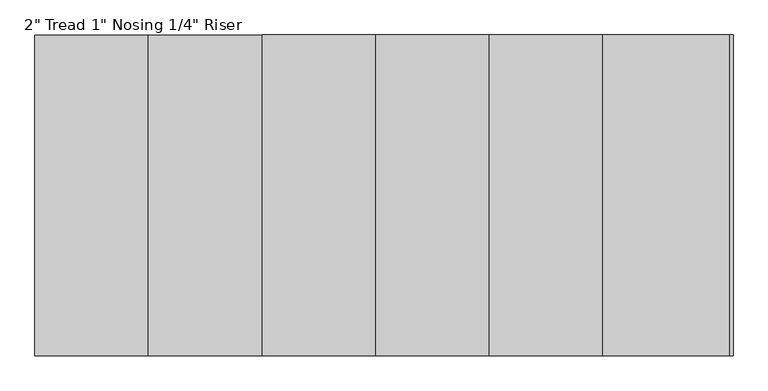
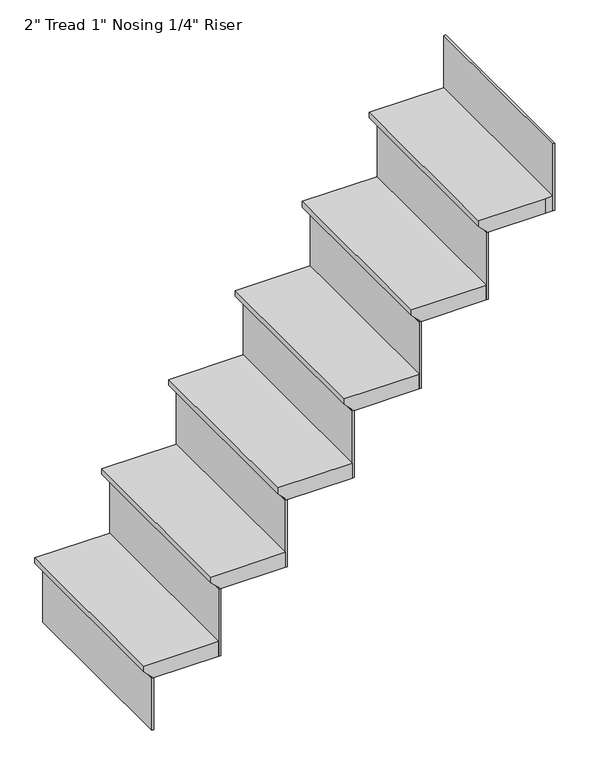
"""IFC4 building model written with IfcOpenShell, lengths in millimetres: stair flight geometry."""

from ifc_helpers import new_model, si_unit, origin, place, context, project, spatial, faceted_brep, source, transform, mapped, element, save


def stair_flight_6b27b35d(model_context):
    return source(origin(), model_context, "Body", "Brep", [
        faceted_brep([(-4591.4237097, 3724.9480625, 209.55), (-4591.4237097, 3724.9480625, 228.6), (-4591.4237097, 4334.5480625, 228.6), (-4591.4237097, 4334.5480625, 209.55), (-4566.0237097, 3724.9480625, 184.15), (-4566.0237097, 4334.5480625, 184.15), (-4350.1237097, 3724.9480625, 228.6), (-4350.1237097, 4334.5480625, 228.6), (-4566.0237097, 4334.5480625, 177.8), (-4350.1237097, 4334.5480625, 177.8), (-4350.1237097, 3724.9480625, 177.8), (-4566.0237097, 3724.9480625, 177.8)], [[[0, 1, 2, 3]], [[4, 0, 3, 5]], [[2, 1, 6, 7]], [[8, 9, 10, 11]], [[2, 7, 9, 8, 5, 3]], [[8, 11, 4, 5]], [[6, 1, 0, 4, 11, 10]], [[7, 6, 10, 9]]]),
        faceted_brep([(-4566.0237097, 3724.9480625, 177.8), (-4566.0237097, 3724.9480625, 0.0), (-4559.6737097, 3724.9480625, 0.0), (-4559.6737097, 3724.9480625, 177.8), (-4566.0237097, 4334.5480625, 177.8), (-4559.6737097, 4334.5480625, 177.8), (-4559.6737097, 4334.5480625, 0.0), (-4566.0237097, 4334.5480625, 0.0)], [[[0, 1, 2, 3]], [[4, 5, 6, 7]], [[1, 0, 4, 7]], [[2, 1, 7, 6]], [[3, 2, 6, 5]], [[0, 3, 5, 4]]]),
        faceted_brep([(-3270.6237097, 3724.9480625, 1549.4), (-3270.6237097, 3724.9480625, 1320.8), (-3264.2737097, 3724.9480625, 1320.8), (-3264.2737097, 3724.9480625, 1549.4), (-3270.6237097, 4334.5480625, 1549.4), (-3264.2737097, 4334.5480625, 1549.4), (-3264.2737097, 4334.5480625, 1320.8), (-3270.6237097, 4334.5480625, 1320.8)], [[[0, 1, 2, 3]], [[4, 5, 6, 7]], [[1, 0, 4, 7]], [[2, 1, 7, 6]], [[3, 2, 6, 5]], [[0, 3, 5, 4]]]),
        faceted_brep([(-4350.1237097, 3724.9480625, 406.4), (-4350.1237097, 3724.9480625, 177.8), (-4343.7737097, 3724.9480625, 177.8), (-4343.7737097, 3724.9480625, 406.4), (-4350.1237097, 4334.5480625, 406.4), (-4343.7737097, 4334.5480625, 406.4), (-4343.7737097, 4334.5480625, 177.8), (-4350.1237097, 4334.5480625, 177.8)], [[[0, 1, 2, 3]], [[4, 5, 6, 7]], [[1, 0, 4, 7]], [[2, 1, 7, 6]], [[3, 2, 6, 5]], [[0, 3, 5, 4]]]),
        faceted_brep([(-4375.5237097, 4334.5480625, 457.2), (-4375.5237097, 3724.9480625, 457.2), (-4134.2237097, 3724.9480625, 457.2), (-4134.2237097, 4334.5480625, 457.2), (-4350.1237097, 4334.5480625, 406.4), (-4134.2237097, 4334.5480625, 406.4), (-4134.2237097, 3724.9480625, 406.4), (-4350.1237097, 3724.9480625, 406.4), (-4350.1237097, 4334.5480625, 412.75), (-4375.5237097, 4334.5480625, 438.15), (-4350.1237097, 3724.9480625, 412.75), (-4375.5237097, 3724.9480625, 438.15)], [[[0, 1, 2, 3]], [[4, 5, 6, 7]], [[0, 3, 5, 4, 8, 9]], [[4, 7, 10, 8]], [[2, 1, 11, 10, 7, 6]], [[3, 2, 6, 5]], [[11, 1, 0, 9]], [[10, 11, 9, 8]]]),
        faceted_brep([(-4134.2237097, 3724.9480625, 635.0), (-4134.2237097, 3724.9480625, 406.4), (-4127.8737097, 3724.9480625, 406.4), (-4127.8737097, 3724.9480625, 635.0), (-4134.2237097, 4334.5480625, 635.0), (-4127.8737097, 4334.5480625, 635.0), (-4127.8737097, 4334.5480625, 406.4), (-4134.2237097, 4334.5480625, 406.4)], [[[0, 1, 2, 3]], [[4, 5, 6, 7]], [[1, 0, 4, 7]], [[2, 1, 7, 6]], [[3, 2, 6, 5]], [[0, 3, 5, 4]]]),
        faceted_brep([(-4159.6237097, 4334.5480625, 685.8), (-4159.6237097, 3724.9480625, 685.8), (-3918.3237097, 3724.9480625, 685.8), (-3918.3237097, 4334.5480625, 685.8), (-4134.2237097, 4334.5480625, 635.0), (-3918.3237097, 4334.5480625, 635.0), (-3918.3237097, 3724.9480625, 635.0), (-4134.2237097, 3724.9480625, 635.0), (-4134.2237097, 4334.5480625, 641.35), (-4159.6237097, 4334.5480625, 666.75), (-4134.2237097, 3724.9480625, 641.35), (-4159.6237097, 3724.9480625, 666.75)], [[[0, 1, 2, 3]], [[4, 5, 6, 7]], [[0, 3, 5, 4, 8, 9]], [[4, 7, 10, 8]], [[2, 1, 11, 10, 7, 6]], [[3, 2, 6, 5]], [[11, 1, 0, 9]], [[10, 11, 9, 8]]]),
        faceted_brep([(-3918.3237097, 3724.9480625, 863.6), (-3918.3237097, 3724.9480625, 635.0), (-3911.9737097, 3724.9480625, 635.0), (-3911.9737097, 3724.9480625, 863.6), (-3918.3237097, 4334.5480625, 863.6), (-3911.9737097, 4334.5480625, 863.6), (-3911.9737097, 4334.5480625, 635.0), (-3918.3237097, 4334.5480625, 635.0)], [[[0, 1, 2, 3]], [[4, 5, 6, 7]], [[1, 0, 4, 7]], [[2, 1, 7, 6]], [[3, 2, 6, 5]], [[0, 3, 5, 4]]]),
        faceted_brep([(-3943.7237097, 4334.5480625, 914.4), (-3943.7237097, 3724.9480625, 914.4), (-3702.4237097, 3724.9480625, 914.4), (-3702.4237097, 4334.5480625, 914.4), (-3918.3237097, 4334.5480625, 863.6), (-3702.4237097, 4334.5480625, 863.6), (-3702.4237097, 3724.9480625, 863.6), (-3918.3237097, 3724.9480625, 863.6), (-3918.3237097, 4334.5480625, 869.95), (-3943.7237097, 4334.5480625, 895.35), (-3918.3237097, 3724.9480625, 869.95), (-3943.7237097, 3724.9480625, 895.35)], [[[0, 1, 2, 3]], [[4, 5, 6, 7]], [[0, 3, 5, 4, 8, 9]], [[4, 7, 10, 8]], [[2, 1, 11, 10, 7, 6]], [[3, 2, 6, 5]], [[11, 1, 0, 9]], [[10, 11, 9, 8]]]),
        faceted_brep([(-3702.4237097, 3724.9480625, 1092.2), (-3702.4237097, 3724.9480625, 863.6), (-3696.0737097, 3724.9480625, 863.6), (-3696.0737097, 3724.9480625, 1092.2), (-3702.4237097, 4334.5480625, 1092.2), (-3696.0737097, 4334.5480625, 1092.2), (-3696.0737097, 4334.5480625, 863.6), (-3702.4237097, 4334.5480625, 863.6)], [[[0, 1, 2, 3]], [[4, 5, 6, 7]], [[1, 0, 4, 7]], [[2, 1, 7, 6]], [[3, 2, 6, 5]], [[0, 3, 5, 4]]]),
        faceted_brep([(-3727.8237097, 4334.5480625, 1143.0), (-3727.8237097, 3724.9480625, 1143.0), (-3486.5237097, 3724.9480625, 1143.0), (-3486.5237097, 4334.5480625, 1143.0), (-3702.4237097, 4334.5480625, 1092.2), (-3486.5237097, 4334.5480625, 1092.2), (-3486.5237097, 3724.9480625, 1092.2), (-3702.4237097, 3724.9480625, 1092.2), (-3702.4237097, 4334.5480625, 1098.55), (-3727.8237097, 4334.5480625, 1123.95), (-3702.4237097, 3724.9480625, 1098.55), (-3727.8237097, 3724.9480625, 1123.95)], [[[0, 1, 2, 3]], [[4, 5, 6, 7]], [[0, 3, 5, 4, 8, 9]], [[4, 7, 10, 8]], [[2, 1, 11, 10, 7, 6]], [[3, 2, 6, 5]], [[11, 1, 0, 9]], [[10, 11, 9, 8]]]),
        faceted_brep([(-3486.5237097, 3724.9480625, 1320.8), (-3486.5237097, 3724.9480625, 1092.2), (-3480.1737097, 3724.9480625, 1092.2), (-3480.1737097, 3724.9480625, 1320.8), (-3486.5237097, 4334.5480625, 1320.8), (-3480.1737097, 4334.5480625, 1320.8), (-3480.1737097, 4334.5480625, 1092.2), (-3486.5237097, 4334.5480625, 1092.2)], [[[0, 1, 2, 3]], [[4, 5, 6, 7]], [[1, 0, 4, 7]], [[2, 1, 7, 6]], [[3, 2, 6, 5]], [[0, 3, 5, 4]]]),
        faceted_brep([(-3511.9237097, 4334.5480625, 1371.6), (-3511.9237097, 3724.9480625, 1371.6), (-3296.0237097, 3724.9480625, 1371.6), (-3270.6237097, 3724.9480625, 1371.6), (-3270.6237097, 4334.5480625, 1371.6), (-3486.5237097, 4334.5480625, 1320.8), (-3270.6237097, 4334.5480625, 1320.8), (-3270.6237097, 3724.9480625, 1320.8), (-3296.0237097, 3724.9480625, 1320.8), (-3486.5237097, 3724.9480625, 1320.8), (-3486.5237097, 4334.5480625, 1327.15), (-3511.9237097, 4334.5480625, 1352.55), (-3486.5237097, 3724.9480625, 1327.15), (-3511.9237097, 3724.9480625, 1352.55)], [[[0, 1, 2, 3, 4]], [[5, 6, 7, 8, 9]], [[0, 4, 6, 5, 10, 11]], [[5, 9, 12, 10]], [[2, 1, 13, 12, 9, 8]], [[3, 2, 8, 7]], [[4, 3, 7, 6]], [[13, 1, 0, 11]], [[12, 13, 11, 10]]]),
    ])


if __name__ == "__main__":
    model = new_model("IFC4")
    model_context = context("Model", 3, world=origin())
    ifc_project = project(units=[si_unit("LENGTHUNIT", "METRE", prefix="MILLI")], contexts=[model_context])
    site = spatial("IfcSite", under=ifc_project)
    building = spatial("IfcBuilding", under=site)
    placement = place(None, origin())
    stair_flight_shape = stair_flight_6b27b35d(model_context)
    element("IfcStairFlight", 1, ObjectType="2\" Tread 1\" Nosing 1/4\" Riser", at=placement, inside=building, context=model_context, shape_type="MappedRepresentation", body=[
        mapped(stair_flight_shape, transform((0.0, 0.0, 0.0), x_axis=(1.0, 0.0, 0.0), y_axis=(0.0, 1.0, 0.0), z_axis=(0.0, 0.0, 1.0))),
    ])
    save(model, "model.ifc")
